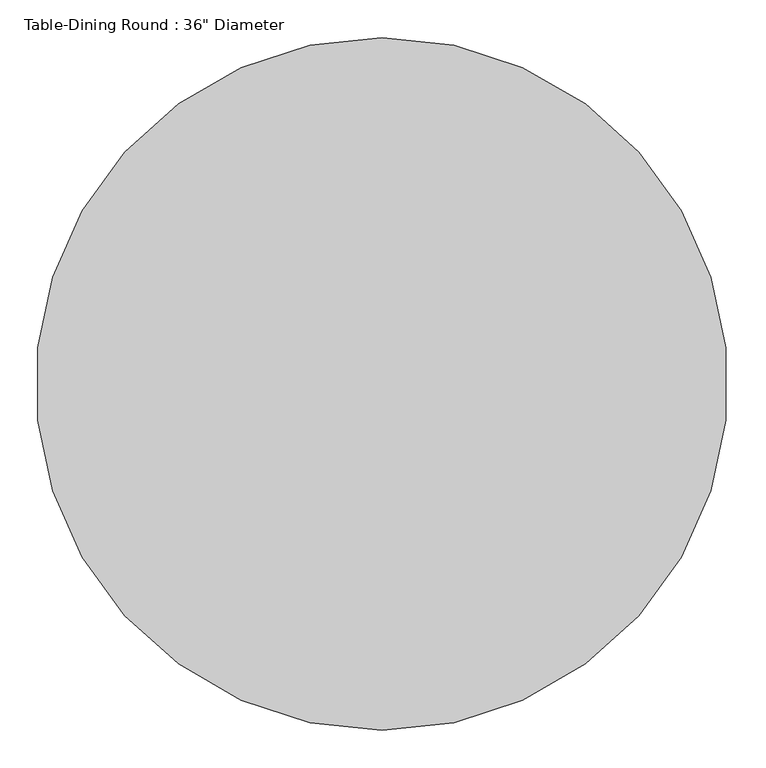
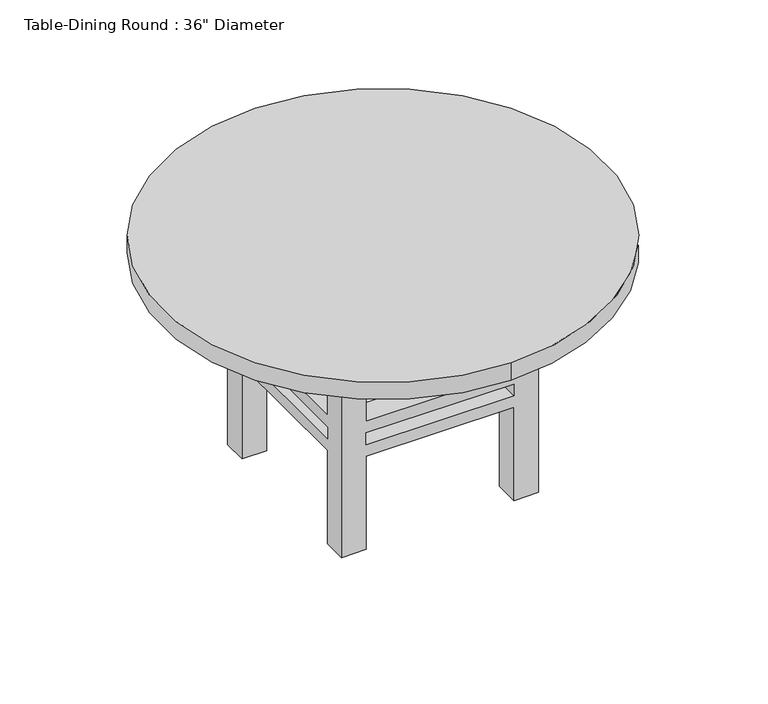
"""IFC4 building model written with IfcOpenShell, lengths in millimetres: furniture geometry."""

from ifc_helpers import new_model, si_unit, point, frame, frame_2d, origin, place, context, project, spatial, polyline, circle_curve, trimmed, segment, composite_curve, outline, extrude, faceted_brep, source, transform, mapped, element, save


def furniture_a1facdee(model_context):
    return source(origin(), model_context, "Body", "SolidModel", [
        faceted_brep([(-48.7180328, 18.3213115, 469.9), (-99.5180328, 18.3213115, 469.9), (-99.5180328, -32.4786885, 469.9), (-48.7180328, -32.4786885, 469.9), (256.0819672, 18.3213115, 469.9), (256.0819672, -32.4786885, 469.9), (306.8819672, -32.4786885, 469.9), (306.8819672, 18.3213115, 469.9), (256.0819672, -388.0786885, 469.9), (306.8819672, -388.0786885, 469.9), (306.8819672, -337.2786885, 469.9), (256.0819672, -337.2786885, 469.9), (-48.7180328, -388.0786885, 469.9), (-48.7180328, -337.2786885, 469.9), (-99.5180328, -337.2786885, 469.9), (-99.5180328, -388.0786885, 469.9), (-48.7180328, 18.3213115, 0.0), (-48.7180328, -32.4786885, 0.0), (-99.5180328, -32.4786885, 0.0), (-99.5180328, 18.3213115, 0.0), (256.0819672, 18.3213115, 0.0), (306.8819672, 18.3213115, 0.0), (306.8819672, -32.4786885, 0.0), (256.0819672, -32.4786885, 0.0), (256.0819672, -388.0786885, 0.0), (256.0819672, -337.2786885, 0.0), (306.8819672, -337.2786885, 0.0), (306.8819672, -388.0786885, 0.0), (-48.7180328, -388.0786885, 0.0), (-99.5180328, -388.0786885, 0.0), (-99.5180328, -337.2786885, 0.0), (-48.7180328, -337.2786885, 0.0), (-48.7180328, 18.3213115, 279.4), (256.0819672, 18.3213115, 279.4), (256.0819672, 18.3213115, 203.2), (-48.7180328, 18.3213115, 203.2), (256.0819672, 18.3213115, 228.6), (256.0819672, 18.3213115, 254.0), (-48.7180328, 18.3213115, 254.0), (-48.7180328, 18.3213115, 228.6), (-99.5180328, -32.4786885, 203.2), (-99.5180328, -337.2786885, 203.2), (-99.5180328, -337.2786885, 279.4), (-99.5180328, -32.4786885, 279.4), (-99.5180328, -32.4786885, 228.6), (-99.5180328, -32.4786885, 254.0), (-99.5180328, -337.2786885, 254.0), (-99.5180328, -337.2786885, 228.6), (-48.7180328, -32.4786885, 279.4), (-48.7180328, -32.4786885, 203.2), (-48.7180328, -32.4786885, 228.6), (-48.7180328, -32.4786885, 254.0), (256.0819672, -32.4786885, 279.4), (256.0819672, -32.4786885, 203.2), (256.0819672, -32.4786885, 228.6), (256.0819672, -32.4786885, 254.0), (306.8819672, -32.4786885, 279.4), (306.8819672, -32.4786885, 203.2), (306.8819672, -32.4786885, 228.6), (306.8819672, -32.4786885, 254.0), (306.8819672, -337.2786885, 279.4), (306.8819672, -337.2786885, 203.2), (306.8819672, -337.2786885, 228.6), (306.8819672, -337.2786885, 254.0), (256.0819672, -388.0786885, 279.4), (-48.7180328, -388.0786885, 279.4), (-48.7180328, -388.0786885, 203.2), (256.0819672, -388.0786885, 203.2), (-48.7180328, -388.0786885, 228.6), (-48.7180328, -388.0786885, 254.0), (256.0819672, -388.0786885, 254.0), (256.0819672, -388.0786885, 228.6), (256.0819672, -337.2786885, 279.4), (256.0819672, -337.2786885, 203.2), (256.0819672, -337.2786885, 228.6), (256.0819672, -337.2786885, 254.0), (-48.7180328, -337.2786885, 279.4), (-48.7180328, -337.2786885, 203.2), (-48.7180328, -337.2786885, 228.6), (-48.7180328, -337.2786885, 254.0)], [[[0, 1, 2, 3]], [[4, 5, 6, 7]], [[8, 9, 10, 11]], [[12, 13, 14, 15]], [[16, 17, 18, 19]], [[20, 21, 22, 23]], [[24, 25, 26, 27]], [[28, 29, 30, 31]], [[1, 0, 32, 33, 4, 7, 21, 20, 34, 35, 16, 19], [36, 37, 38, 39]], [[2, 1, 19, 18, 40, 41, 30, 29, 15, 14, 42, 43], [44, 45, 46, 47]], [[3, 2, 43, 48]], [[18, 17, 49, 40]], [[44, 50, 51, 45]], [[0, 3, 48, 32]], [[17, 16, 35, 49]], [[50, 39, 38, 51]], [[5, 4, 33, 52]], [[20, 23, 53, 34]], [[36, 54, 55, 37]], [[6, 5, 52, 56]], [[23, 22, 57, 53]], [[54, 58, 59, 55]], [[21, 7, 6, 56, 60, 10, 9, 27, 26, 61, 57, 22], [62, 63, 59, 58]], [[27, 9, 8, 64, 65, 12, 15, 29, 28, 66, 67, 24], [68, 69, 70, 71]], [[11, 10, 60, 72]], [[26, 25, 73, 61]], [[62, 74, 75, 63]], [[8, 11, 72, 64]], [[25, 24, 67, 73]], [[74, 71, 70, 75]], [[13, 12, 65, 76]], [[28, 31, 77, 66]], [[68, 78, 79, 69]], [[14, 13, 76, 42]], [[31, 30, 41, 77]], [[78, 47, 46, 79]], [[54, 74, 62, 58]], [[74, 78, 68, 71]], [[78, 50, 44, 47]], [[50, 54, 36, 39]], [[53, 49, 35, 34]], [[49, 77, 41, 40]], [[77, 73, 67, 66]], [[73, 53, 57, 61]], [[74, 54, 53, 73]], [[78, 74, 73, 77]], [[50, 78, 77, 49]], [[54, 50, 49, 53]], [[52, 72, 60, 56]], [[72, 76, 65, 64]], [[76, 48, 43, 42]], [[48, 52, 33, 32]], [[55, 51, 38, 37]], [[51, 79, 46, 45]], [[79, 75, 70, 69]], [[75, 55, 59, 63]], [[72, 52, 55, 75]], [[76, 72, 75, 79]], [[48, 76, 79, 51]], [[52, 48, 51, 55]]]),
        extrude(outline(polyline([(332.2819672, 43.7213115), (332.2819672, -413.4786885), (-124.9180328, -413.4786885), (-124.9180328, 43.7213115), (332.2819672, 43.7213115)]), holes=[polyline([(306.8819672, 18.3213115), (-99.5180328, 18.3213115), (-99.5180328, -388.0786885), (306.8819672, -388.0786885), (306.8819672, 18.3213115)])]), frame((0.0, 0.0, 393.7), z_axis=(0.0, 0.0, 1.0), x_axis=(1.0, 0.0, 0.0)), (0.0, 0.0, 1.0), 76.2),
        extrude(outline(composite_curve([segment(trimmed(circle_curve(frame_2d((103.6819672, -184.8786885)), 457.2), [point((103.6819672, -642.0786885))], [point((103.6819672, 272.3213115))], False, "CARTESIAN"), True, "CONTINUOUS"), segment(trimmed(circle_curve(frame_2d((103.6819672, -184.8786885)), 457.2), [point((103.6819672, 272.3213115))], [point((103.6819672, -642.0786885))], False, "CARTESIAN"), True, "CONTINUOUS")], self_intersect=False)), frame((0.0, 0.0, 469.9), z_axis=(0.0, 0.0, 1.0), x_axis=(1.0, 0.0, 0.0)), (0.0, 0.0, 1.0), 38.1),
    ])


if __name__ == "__main__":
    model = new_model("IFC4")
    model_context = context("Model", 3, world=origin())
    ifc_project = project(units=[si_unit("LENGTHUNIT", "METRE", prefix="MILLI")], contexts=[model_context])
    site = spatial("IfcSite", under=ifc_project)
    building = spatial("IfcBuilding", under=site)
    placement = place(None, origin())
    furniture_shape = furniture_a1facdee(model_context)
    element("IfcFurniture", 1, ObjectType="Table-Dining Round : 36\" Diameter", at=placement, inside=building, context=model_context, shape_type="MappedRepresentation", body=[
        mapped(furniture_shape, transform((0.0, 0.0, 0.0), x_axis=(1.0, 0.0, 0.0), y_axis=(0.0, 1.0, 0.0), z_axis=(0.0, 0.0, 1.0))),
    ])
    save(model, "model.ifc")

# Revit data of these elements
# Type "Table-Dining Round : 36\" Diameter"
#   Assembly Code = "E2020200"
#   Diameter = 3' - 0"
#   Height = 1' - 8"
#   Base Material = Pine
#   Top Material = Laminate, Linen, Matte
#   Default Elevation = 0
# Element 1 (IfcFurniture, "Table-Dining Round : 36\" Diameter")
#   Materials on its faces: "Pine", "Laminate, Linen, Matte"
# Materials
#   "Pine": class "Wood", colour RGB 223 192 134, transparency 0, Description = "Pinus Echinata", Cost = 0
#   "Laminate, Linen, Matte": class "Plastic", colour RGB 249 239 230, transparency 0, Description = "Plastic Laminate - Linen, Matte", Cost = 0
